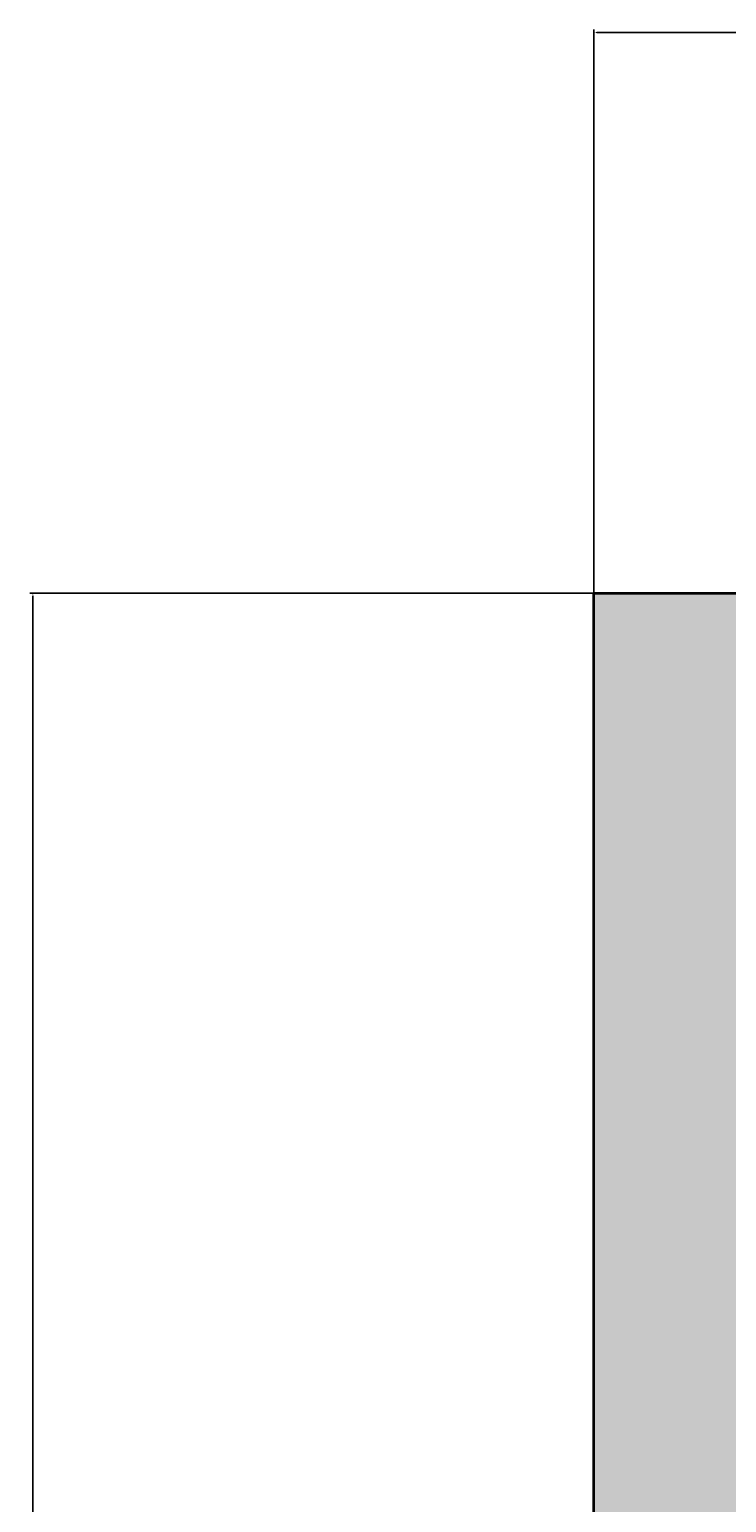
# Model space of a CAD drawing. Units: inches. Extents: x 2070 to 4408, y 1595 to 4269.
# Tile 12 of 20: x 2070 to 2111, y 2238 to 2325. Entities that reach past the tile are written whole.
import ezdxf

# ---------------------------------------------------------------- set-up
doc = ezdxf.new("R2010")
doc.units = ezdxf.units.IN
doc.layers.add('A-ANNO-DIMS', color=2, linetype='Continuous', lineweight=18)
doc.layers.add('A-WALL', color=7, linetype='Continuous', lineweight=35)
doc.layers.add('A-WALL-PATT', color=18, linetype='Continuous', lineweight=13, true_color=0x000000)
doc.styles.get("Standard").update_dxf_attribs({"font": 'arial.ttf'})
doc.dimstyles.get("Standard").update_dxf_attribs({"dimtxt": 0.18, "dimasz": 0.18, "dimexe": 0.18, "dimexo": 0.0625, "dimgap": 0.09, "dimtad": 0, "dimtih": 1, "dimtoh": 1, "dimdec": 4, "dimzin": 0, "dimdsep": 46, "dimtxsty": 'Standard', "dimcen": 0.09, "dimadec": 0, "dimazin": 0, "dimtfac": 1, "dimtdec": 4, "dimtofl": 0, "dimtmove": 0, "dimatfit": 3, "dimfxl": 1, "dimtolj": 1, "dimtzin": 0, "dimarcsym": 0})

# ---------------------------------------------------------------- blocks, each defined once
blk = doc.blocks.new('*D23')
at = {"layer": 'A-ANNO-DIMS', "color": 0, "lineweight": -2, "transparency": 16777216}
for p, q in [((2103.196, 2291.462), (2103.196, 2324.76)), ((2455.196, 2291.462), (2455.196, 2324.76)), ((2103.376, 2324.579), (2278.908, 2324.579)), ((2455.016, 2324.579), (2279.484, 2324.579))]:
    blk.add_line(p, q, dxfattribs=at)
at = {"layer": 'A-ANNO-DIMS', "color": 0, "transparency": 16777216}
for points in [[(2103.376, 2324.61), (2103.376, 2324.55), (2103.196, 2324.579)], [(2455.016, 2324.61), (2455.016, 2324.55), (2455.196, 2324.579)]]:
    blk.add_solid(points, dxfattribs=at)
at = {"layer": 'Defpoints', "color": 0, "transparency": 16777216}
for p in [(2455.196, 2324.579), (2103.196, 2291.399), (2455.196, 2291.399)]:
    blk.add_point(p, dxfattribs=at)
at = {"layer": 'A-ANNO-DIMS', "color": 0, "transparency": 16777216, "insert": (2279.196, 2324.579), "char_height": 0.18, "attachment_point": 5}
blk.add_mtext('\\A1;352', dxfattribs=at)
blk = doc.blocks.new('*D24')
at = {"layer": 'A-ANNO-DIMS', "color": 0, "lineweight": -2, "transparency": 16777216}
for p, q in [((2103.133, 2291.4), (2069.836, 2291.4)), ((2070.016, 2291.22), (2070.016, 1960.081)), ((2070.016, 1628.58), (2070.016, 1959.718)), ((2336.133, 1628.4), (2069.836, 1628.4))]:
    blk.add_line(p, q, dxfattribs=at)
at = {"layer": 'A-ANNO-DIMS', "color": 0, "transparency": 16777216}
for points in [[(2069.986, 2291.22), (2070.046, 2291.22), (2070.016, 2291.4)], [(2069.986, 1628.58), (2070.046, 1628.58), (2070.016, 1628.4)]]:
    blk.add_solid(points, dxfattribs=at)
at = {"layer": 'Defpoints', "color": 0, "transparency": 16777216}
for p in [(2070.016, 2291.4), (2103.196, 2291.4), (2336.196, 1628.4)]:
    blk.add_point(p, dxfattribs=at)
at = {"layer": 'A-ANNO-DIMS', "color": 0, "transparency": 16777216, "insert": (2070.016, 1959.899), "char_height": 0.18, "attachment_point": 5}
blk.add_mtext('\\A1;663', dxfattribs=at)

msp = doc.modelspace()

# ---------------------------------------------------------------- hatches: boundary and pattern name
at = {"layer": 'A-WALL-PATT'}
h = msp.add_hatch(color=256, dxfattribs=at)
h.dxf.hatch_style = 1
h.paths.add_polyline_path([(2346.196, 2218.3995), (2346.196, 2282.3995), (2340.196, 2282.3995), (2340.196, 2212.3995), (2345.5866, 2212.3995), (2346.196, 2212.3995)], flags=0)
h.paths.add_polyline_path([(2245.196, 2282.3995), (2239.196, 2282.3995), (2239.196, 2186.3995), (2244.5866, 2186.3995), (2245.196, 2186.3995)], flags=0)
h.paths.add_polyline_path([(2340.196, 2230.6455), (2245.196, 2230.6455), (2245.196, 2224.6455), (2340.196, 2224.6455)], flags=0)
h.paths.add_polyline_path([(2245.196, 2150.3995), (2239.196, 2150.3995), (2164.4362, 2150.3995), (2164.4362, 2144.3995), (2239.196, 2144.3995), (2239.196, 2086.3995), (2239.196, 2067.2711), (2244.5866, 2067.2711), (2245.196, 2067.2711), (2245.196, 2144.3995)], flags=0)
h.paths.add_polyline_path([(2346.196, 2176.3995), (2340.196, 2176.3995), (2340.196, 2086.3995), (2346.196, 2086.3995), (2346.196, 2125.318)], flags=0)
h.paths.add_polyline_path([(2446.196, 2086.3995), (2346.196, 2086.3995), (2340.196, 2086.3995), (2340.196, 2080.3995), (2446.196, 2080.3995)], flags=0)
h.paths.add_polyline_path([(2455.196, 2291.3995), (2103.196, 2291.3995), (2103.196, 1699.3995), (2336.196, 1699.3995), (2336.196, 1628.3995), (2345.196, 1628.3995), (2446.196, 1628.3995), (2454.8846, 1628.3995), (2454.8846, 1699.3995)])
h.paths.add_polyline_path([(2446.196, 2282.3995), (2446.196, 2218.3995), (2446.196, 2212.3995), (2446.196, 2086.3995), (2446.196, 2080.3995), (2446.196, 1708.3995), (2446.196, 1637.3995), (2345.196, 1637.3995), (2345.196, 1699.3995), (2345.196, 1708.3995), (2336.196, 1708.3995), (2112.196, 1708.3995), (2112.196, 2282.3995), (2239.196, 2282.3995), (2245.196, 2282.3995), (2356.196, 2282.3995)], flags=16)
h.paths.add_polyline_path([(2245.196, 2150.3995), (2245.196, 2144.3995), (2245.196, 2067.2711), (2244.5866, 2067.2711), (2239.196, 2067.2711), (2239.196, 2065.6988), (2203.2929, 2065.6988, 0.4014527), (2239.196, 2031.3337), (2244.5866, 2031.3337), (2245.196, 2031.2711), (2245.196, 1924.1525), (2239.196, 1924.1525), (2239.196, 1922.5803), (2203.2929, 1922.5803, 0.4014527), (2239.196, 1888.2151), (2244.5866, 1888.2151), (2245.196, 1888.1525), (2245.196, 1748.3995), (2339.196, 1748.4621, -0.4014527), (2303.2929, 1782.8272), (2303.2585, 1782.8272), (2303.2585, 1784.3995), (2339.196, 1784.3995), (2339.196, 1877.2067), (2291.196, 1877.2067), (2291.196, 1883.2067), (2291.196, 1946.3995), (2291.196, 1952.3995), (2291.196, 2086.3995), (2297.196, 2086.3995), (2302.196, 2086.3995), (2302.196, 2081.0259), (2303.7633, 2081.0259), (2303.7633, 2080.3995), (2338.0148, 2080.3995, 0.0043713), (2338.0203, 2081.0259), (2338.0203, 2086.3995), (2340.196, 2086.3995), (2340.196, 2176.4621), (2345.5866, 2176.4621, 0.4014527), (2381.4896, 2210.8272), (2345.5866, 2210.8272), (2345.5866, 2212.3995), (2340.196, 2212.3995), (2340.196, 2224.6455), (2245.196, 2224.6455), (2245.196, 2186.3995), (2244.5866, 2186.3995), (2239.196, 2186.3995), (2239.196, 2184.8272), (2203.2929, 2184.8272, 0.4014527), (2239.196, 2150.4621), (2244.5866, 2150.4621)], flags=0)
h.paths.add_polyline_path([(2346.196, 2282.3995), (2346.196, 2218.3995), (2377.1813, 2218.3995), (2377.1813, 2212.3995), (2346.196, 2212.3995), (2345.5866, 2212.3995), (2340.196, 2212.3995), (2340.196, 2224.6455), (2245.196, 2224.6455), (2245.196, 2230.6455), (2245.196, 2282.3995), (2292.696, 2256.5225), (2340.196, 2282.3995)], flags=0)
h.paths.add_polyline_path([(2346.196, 2086.3995), (2340.196, 2086.3995), (2340.196, 2080.3995), (2446.196, 2080.3995), (2431.196, 2016.3995), (2446.196, 1952.3995), (2412.196, 1952.3995), (2412.196, 2080.3995), (2340.196, 2080.3995), (2340.196, 2086.3995), (2340.196, 2176.3995), (2346.196, 2176.3995), (2346.196, 2125.318)], flags=0)
h.paths.add_polyline_path([(2186.508, 2270.0471, -0.0375529), (2186.9712, 2269.8581), (2186.9164, 2270.112, -0.0275912)], flags=0)
h.paths.add_polyline_path([(2183.955, 2273.7766, 1), (2188.2945, 2273.7766, 1)], flags=0)
h.paths.add_polyline_path([(2142.5261, 2274.6158, -0.0370754), (2142.5672, 2275.1696), (2142.5672, 2276.826), (2119.8759, 2276.826), (2119.8759, 2263.0962), (2140.4332, 2263.0962), (2142.5672, 2263.0962), (2142.5672, 2274.0621, -0.0370754)], flags=0)
h.paths.add_polyline_path([(2209.8974, 2263.0962), (2209.8974, 2262.2079), (2190.8042, 2262.2079), (2190.8042, 2263.0962)], flags=0)
h.paths.add_polyline_path([(2210.6382, 2276.1833), (2210.6382, 2263.9844), (2190.2185, 2263.9844), (2190.2185, 2276.1833)], flags=0)
h.paths.add_polyline_path([(2188.4362, 2273.7766, -1), (2183.8133, 2273.7766, -1)], flags=0)
h.paths.add_polyline_path([(2245.196, 2150.3995), (2245.196, 2144.3995), (2245.196, 2067.2711), (2239.196, 2067.2711), (2239.196, 2080.3995), (2172.196, 2080.3995), (2172.196, 2000.3995), (2239.196, 2000.3995), (2239.196, 1940.3995), (2159.0187, 1940.3995), (2123.0187, 1940.3995), (2112.196, 1940.3995), (2112.196, 1946.3995), (2123.0187, 1946.3995), (2123.0187, 1982.2238), (2124.586, 1982.2238), (2124.586, 1982.1895, -0.4014527), (2158.8429, 1946.3995), (2159.0187, 1946.3995), (2239.196, 1946.3995), (2239.196, 1994.3995), (2112.196, 1994.3995), (2112.196, 2000.3995), (2139.196, 2040.3995), (2112.196, 2080.3995), (2112.196, 2086.3995), (2239.196, 2086.3995), (2239.196, 2144.3995), (2209.5809, 2144.3995), (2209.5809, 2136.3995), (2203.0809, 2136.3995), (2205.0809, 2130.3996, -0.7025712), (2199.081, 2116.3995, -0.7025621), (2193.0809, 2130.3994), (2195.0809, 2136.3995), (2192.0809, 2136.3995), (2192.0809, 2134.8995), (2189.0809, 2134.8995), (2189.0809, 2135.8995), (2191.0809, 2135.8995), (2191.0809, 2136.3995), (2188.5809, 2136.3995), (2188.5809, 2144.3995), (2164.2481, 2144.3995, -0.3938585), (2130.0035, 2109.5491), (2130.0035, 2109.5147), (2128.4362, 2109.5147), (2128.4362, 2144.3995), (2112.196, 2144.3995), (2112.196, 2150.3995), (2128.4362, 2150.3995), (2128.4362, 2150.7127), (2164.4362, 2150.7127), (2164.4362, 2150.3995), (2239.196, 2150.3995)], flags=0)
h.paths.add_polyline_path([(2188.2075, 2266.8735), (2188.2075, 2211.8632, -0.4142136), (2185.4833, 2209.1391), (2146.7995, 2209.1391, -0.4142136), (2144.0754, 2211.8632), (2144.0754, 2266.8735, -0.4142136), (2146.7995, 2269.5976), (2185.4833, 2269.5976, -0.4142136)], flags=0)
h.paths.add_polyline_path([(2185.0844, 2273.7766, -1), (2187.1651, 2273.7766, -1)], flags=0)
h.paths.add_polyline_path([(2182.0486, 2259.2932), (2168.0953, 2259.2932), (2168.0953, 2260.8424), (2163.7261, 2260.8424), (2163.7261, 2259.2932), (2149.7727, 2259.2932), (2149.7727, 2266.3352), (2163.7261, 2266.3352), (2163.7261, 2261.9839), (2168.0953, 2261.9839), (2168.0953, 2266.3352), (2182.0486, 2266.3352)], flags=0)
h.paths.add_polyline_path([(2148.2585, 2250.2051), (2153.0615, 2241.8861, 0.3980705)], flags=0)
h.paths.add_polyline_path([(2162.7572, 2247.2885), (2153.1461, 2241.7396), (2148.1083, 2250.4653), (2157.7194, 2256.0142)], flags=0)
h.paths.add_polyline_path([(2162.6726, 2247.4351, -0.392862), (2157.8415, 2255.6313), (2157.6431, 2255.6313), (2157.8696, 2255.7541)], flags=0)
h.paths.add_polyline_path([(2164.2604, 2145.339), (2164.4362, 2144.3995), (2164.4362, 2150.3995), (2164.2604, 2150.7127)], flags=0)
h.paths.add_polyline_path([(2208.5809, 2142.6495), (2208.5809, 2138.3995, -0.4142136), (2207.8309, 2137.3995), (2190.5809, 2137.3995, -0.4142136), (2189.5809, 2138.1495), (2189.5809, 2142.3995, -0.4142136), (2190.3309, 2143.3995), (2207.5809, 2143.3995, -0.4142136)], flags=0)
h.paths.add_polyline_path([(2147.957, 2229.9119), (2154.7494, 2223.1195, 0.3980705)], flags=0)
h.paths.add_polyline_path([(2162.7165, 2230.8473), (2154.8691, 2222.9998), (2147.7446, 2230.1244), (2155.592, 2237.9718)], flags=0)
h.paths.add_polyline_path([(2162.5969, 2230.9669, -0.3980705), (2155.8044, 2237.7594)], flags=0)
h.paths.add_polyline_path([(2391.8776, 2049.9192), (2408.5766, 2049.9192), (2408.5766, 2033.2202), (2408.5766, 1983.123), (2408.5766, 1966.4239), (2391.8776, 1966.4239), (2391.8776, 1983.123), (2341.7804, 1983.123), (2341.7804, 2033.2202), (2391.8776, 2033.2202)], flags=0)
h.paths.add_polyline_path([(2144.1055, 2274.6158, 1), (2148.445, 2274.6158, 1)], flags=0)
h.paths.add_polyline_path([(2148.5867, 2274.6158, -1), (2143.9638, 2274.6158, -1)], flags=0)
h.paths.add_polyline_path([(2145.2349, 2274.6158, -1), (2147.3156, 2274.6158, -1)], flags=0)
edge = h.paths.add_edge_path(flags=0)
edge.add_ellipse((2400.5951, 2040.9436), major_axis=(-4.5109, 0), ratio=0.9754478, start_angle=180, end_angle=270, ccw=False)
edge.add_ellipse((2400.5951, 2040.9436), major_axis=(-4.5109, 0), ratio=0.9754478, start_angle=90, end_angle=180, ccw=False)
edge.add_ellipse((2400.5951, 2040.9436), major_axis=(-4.5109, 0), ratio=0.9754478, start_angle=0, end_angle=90, ccw=False)
edge.add_ellipse((2400.5951, 2040.9436), major_axis=(-4.5109, 0), ratio=0.9754478, start_angle=270, end_angle=360, ccw=False)
h.paths.add_polyline_path([(2199.0809, 2117.3995, -0.7345297), (2195.0809, 2130.3995), (2203.081, 2130.3995, -0.7345333)], flags=0)
h.paths.add_polyline_path([(2141.9147, 2276.0353), (2141.9147, 2263.9844), (2120.4685, 2263.9844), (2120.4685, 2276.0353)], flags=0)
h.paths.add_polyline_path([(2138.4481, 2273.4072), (2138.4481, 2266.7226), (2133.2801, 2266.7226), (2133.2801, 2273.4072)], flags=0)
h.paths.add_polyline_path([(2137.9691, 2272.9175), (2137.9691, 2272.204), (2135.4229, 2272.204), (2135.4229, 2271.6329), (2135.3221, 2270.1051), (2135.3221, 2269.0265), (2135.4229, 2268.6811), (2135.4229, 2267.2011), (2133.7212, 2267.2011), (2133.7212, 2268.6811), (2133.7983, 2269.9587), (2133.7983, 2271.2758), (2133.7212, 2271.6329), (2133.7212, 2273.0065), (2135.717, 2273.0065), (2135.717, 2272.9175)], flags=0)
h.paths.add_polyline_path([(2137.9215, 2271.8264), (2137.9215, 2271.3786), (2137.5182, 2271.3786), (2136.9355, 2271.3786), (2136.3529, 2271.3786), (2135.7703, 2271.3786), (2135.7703, 2271.8264), (2136.1736, 2271.8264), (2136.7562, 2271.8264), (2137.3389, 2271.8264)], flags=0)
h.paths.add_polyline_path([(2137.9215, 2271.692), (2137.5182, 2271.692), (2136.9355, 2271.513), (2137.3389, 2271.513)], flags=0)
h.paths.add_polyline_path([(2136.3529, 2271.692), (2135.7703, 2271.513), (2136.1736, 2271.513), (2136.7562, 2271.692)], flags=0)
h.paths.add_polyline_path([(2137.9215, 2271.513), (2137.5182, 2271.513), (2136.7562, 2271.747), (2136.7562, 2271.692), (2137.3389, 2271.692)], flags=0)
h.paths.add_polyline_path([(2137.8207, 2270.4664), (2137.8207, 2270.0971), (2137.8207, 2269.627), (2137.8207, 2269.1569), (2137.8207, 2268.6868), (2137.3837, 2268.6868), (2136.6442, 2268.6868), (2135.9271, 2268.6868), (2135.9271, 2269.0562), (2135.9271, 2269.5263), (2135.9271, 2269.9963), (2135.9271, 2270.4664), (2136.3641, 2270.4664), (2137.0812, 2270.4664)], flags=0)
h.paths.add_polyline_path([(2137.3837, 2269.627), (2137.8207, 2269.627), (2137.8207, 2269.5263), (2137.3837, 2269.5263), (2137.3837, 2269.1569), (2137.8207, 2269.1569), (2137.3837, 2269.0562), (2137.3837, 2268.6868), (2137.0812, 2268.6868), (2137.0812, 2269.0562), (2136.6442, 2269.0562), (2136.6442, 2268.6868), (2136.3641, 2268.6868), (2136.3641, 2269.0562), (2135.9271, 2269.0562), (2135.9271, 2269.1569), (2136.3641, 2269.1569), (2136.3641, 2269.5263), (2135.9271, 2269.5263), (2135.9271, 2269.627), (2136.3641, 2269.627), (2136.3641, 2269.9963), (2135.9271, 2269.9963), (2136.3641, 2270.0971), (2136.3641, 2270.4664), (2136.6442, 2270.4664), (2136.6442, 2270.0971), (2137.0812, 2270.0971), (2137.0812, 2270.4664), (2137.3837, 2270.4664), (2137.3837, 2270.0971), (2137.8207, 2270.0971), (2137.3837, 2269.9963)], flags=0)
h.paths.add_polyline_path([(2137.5182, 2271.8264), (2137.5182, 2271.692), (2137.3389, 2271.3786), (2137.3389, 2271.513)], flags=0)
h.paths.add_polyline_path([(2137.8179, 2267.8138), (2137.8179, 2267.6879), (2137.1876, 2267.6879), (2136.4733, 2267.6879), (2135.759, 2267.6879), (2135.759, 2267.8138), (2136.3893, 2267.8138), (2137.1036, 2267.8138)], flags=0)
h.paths.add_polyline_path([(2137.0812, 2269.9963), (2137.0812, 2269.627), (2137.0812, 2269.1569), (2136.6442, 2269.1569), (2136.6442, 2269.5263), (2136.6442, 2269.9963)], flags=0)
h.paths.add_polyline_path([(2136.3529, 2271.8264), (2136.3529, 2271.692), (2136.1736, 2271.3786), (2136.1736, 2271.513)], flags=0)
h.paths.add_polyline_path([(2136.4733, 2267.8138), (2136.4733, 2267.6879), (2136.3893, 2267.6879), (2136.3893, 2267.8138)], flags=0)
h.paths.add_polyline_path([(2407.9087, 2032.5522), (2407.9087, 1983.7909), (2359.81, 1983.7909, -0.0091279), (2359.0575, 1983.7909), (2342.4483, 1983.7909), (2342.4483, 2032.5522)], flags=0)
h.paths.add_polyline_path([(2389.1838, 2023.1358), (2353.7856, 2023.1358), (2353.7856, 1985.4867, -0.0921038), (2350.2788, 1988.655), (2350.2788, 2026.6426), (2389.1838, 2026.6426)], flags=0)
h.paths.add_polyline_path([(2352.6166, 2024.3048), (2351.4477, 2024.3048), (2351.4477, 2025.4737), (2352.6166, 2025.4737)], flags=0)
h.paths.add_polyline_path([(2399.6319, 2026.7589), (2404.3661, 2026.7589, -0.4142136), (2407.0379, 2024.087), (2407.0379, 2013.4908, -0.4142136), (2404.3661, 2010.819), (2399.6319, 2010.819, -0.4142136), (2396.96, 2013.4908), (2396.96, 2024.087, -0.4142136)], flags=0)
h.paths.add_polyline_path([(2399.6319, 2026.0909), (2404.3661, 2026.0909, -0.4142136), (2406.37, 2024.087), (2406.37, 2013.4908, -0.4142136), (2404.3661, 2011.487), (2399.6319, 2011.487, -0.4142136), (2397.628, 2013.4908), (2397.628, 2024.087, -0.4142136)], flags=0)
h.paths.add_polyline_path([(2399.6319, 2002.3217), (2404.3661, 2002.3217, -0.4142136), (2407.0379, 1999.6498), (2407.0379, 1989.0536, -0.4142136), (2404.3661, 1986.3818), (2399.6319, 1986.3818, -0.4142136), (2396.96, 1989.0536), (2396.96, 1999.6498, -0.4142136)], flags=0)
h.paths.add_polyline_path([(2399.6319, 2001.6537), (2404.3661, 2001.6537, -0.4142136), (2406.37, 1999.6498), (2406.37, 1989.0536, -0.4142136), (2404.3661, 1987.0497), (2399.6319, 1987.0497, -0.4142136), (2397.628, 1989.0536), (2397.628, 1999.6498, -0.4142136)], flags=0)
edge = h.paths.add_edge_path(flags=0)
edge.add_ellipse((2400.5951, 1975.3996), major_axis=(-4.5109, 0), ratio=0.9754478, start_angle=-180, end_angle=-90, ccw=False)
edge.add_ellipse((2400.5951, 1975.3996), major_axis=(-4.5109, 0), ratio=0.9754478, start_angle=90, end_angle=180, ccw=False)
edge.add_ellipse((2400.5951, 1975.3996), major_axis=(-4.5109, 0), ratio=0.9754478, start_angle=0, end_angle=90, ccw=False)
edge.add_ellipse((2400.5951, 1975.3996), major_axis=(-4.5109, 0), ratio=0.9754478, start_angle=-90, end_angle=0, ccw=False)
h.paths.add_polyline_path([(2345.196, 1910.3995), (2366.4386, 1910.3995), (2366.4386, 1925.4555), (2392.3856, 1925.4555), (2392.3856, 1933.5025), (2400.1399, 1925.4555), (2392.3856, 1919.8795), (2392.3856, 1925.4555), (2366.4386, 1925.4555), (2366.4386, 1910.3995), (2381.196, 1910.3995), (2405.196, 1910.3995), (2405.196, 1898.3995), (2446.196, 1898.3995), (2446.196, 1886.3995), (2405.196, 1886.3995), (2405.196, 1874.3995), (2446.196, 1874.3995), (2446.196, 1862.3995), (2405.196, 1862.3995), (2405.196, 1850.3995), (2446.196, 1850.3995), (2446.196, 1838.3995), (2405.196, 1838.3995), (2405.196, 1826.3995), (2446.196, 1826.3995), (2446.196, 1814.3995), (2405.196, 1814.3995), (2405.196, 1802.3995), (2446.196, 1802.3995), (2446.196, 1798.3995), (2446.196, 1792.3995), (2405.196, 1792.3995), (2405.196, 1910.3995), (2381.196, 1910.3995), (2381.196, 1792.3995), (2345.196, 1792.3995)], flags=0)
h.paths.add_polyline_path([(2333.0944, 1863.3993, -0.4142136), (2334.7225, 1861.7712), (2334.7225, 1859.329), (2335.2653, 1859.329, -0.4142136), (2337.4361, 1857.1582), (2337.4361, 1843.862, -0.4142136), (2335.2653, 1841.6911, -0.4142136), (2337.4361, 1839.5203), (2337.4361, 1827.5808, -0.4142136), (2335.2653, 1825.41, -0.4142136), (2337.4361, 1823.2392), (2337.4361, 1808.5862, -0.4142136), (2335.2653, 1806.4153), (2334.7225, 1806.4153), (2334.7225, 1803.9732, -0.4142136), (2333.0944, 1802.3451), (2317.356, 1802.3451), (2317.0846, 1802.3451, -0.4142136), (2315.7279, 1803.7018), (2315.7279, 1803.8646), (2313.8284, 1803.8646, -0.4142136), (2311.6576, 1806.0354), (2311.6576, 1823.2015, -0.395976), (2313.6834, 1825.3765, -0.433848), (2311.6576, 1827.2718), (2311.6576, 1839.761, -0.4142136), (2313.5571, 1841.6604), (2313.8284, 1841.6604), (2333.8159, 1841.6604, -0.0421362), (2334.1798, 1841.6911, -0.4142136), (2332.009, 1843.862), (2332.009, 1857.1582, -0.4142136), (2334.1798, 1859.329), (2317.356, 1859.329), (2317.0846, 1859.329, -0.4142136), (2315.7279, 1860.6858), (2315.7279, 1862.0426, -0.4142136), (2317.0846, 1863.3993), (2317.356, 1863.3993)], flags=0)
h.paths.add_polyline_path([(2208.8475, 1848.9818), (2208.8475, 1840.9741, -0.4142136), (2207.0458, 1839.1724), (2206.5453, 1839.1721), (2206.5453, 1838.7218, -0.4098586), (2204.7704, 1836.9203), (2183.7501, 1836.9203, -0.418582), (2181.9216, 1838.7218), (2181.9216, 1839.1721), (2181.421, 1839.1724, -0.4142136), (2179.6193, 1840.9741), (2179.6193, 1848.6817, -0.4406442), (2185.1126, 1854.9874), (2203.3852, 1854.9874, -0.4570796)], flags=0)
h.paths.add_polyline_path([(2204.243, 1848.4815), (2204.243, 1848.4815, 0.4172533), (2202.2204, 1850.4833), (2186.2049, 1850.4833, 0.4111805), (2184.2237, 1848.4815), (2184.2237, 1848.4815, -0.4111807), (2186.2049, 1850.4833), (2202.2204, 1850.4833, -0.4172531)], flags=0)
h.paths.add_polyline_path([(2234.7177, 1830.228), (2234.7176, 1781.6047, -0.4142136), (2233.4381, 1780.3252), (2218.6064, 1780.3252, -0.4142136), (2217.8387, 1781.0929), (2217.8387, 1783.3961, -0.4142136), (2218.6064, 1784.1639), (2218.6065, 1796.9595, -0.4142136), (2219.886, 1798.239, -0.4142136), (2218.6065, 1799.5186), (2218.6065, 1812.3142, -0.4142136), (2219.8861, 1813.5938, -0.4142136), (2218.6065, 1814.8733), (2218.6065, 1827.6689, -0.4142136), (2217.8388, 1828.4367), (2217.8388, 1830.7399, -0.4142136), (2218.6065, 1831.5076), (2233.4382, 1831.5076, -0.4142136)], flags=0)
h.paths.add_polyline_path([(2230.6344, 1827.6689, -0.4142136), (2231.4021, 1826.9012), (2231.4021, 1784.9316, -0.4142136), (2230.6343, 1784.1639), (2221.1853, 1784.1639), (2221.1853, 1827.6689)], flags=0)
h.paths.add_polyline_path([(2222.7208, 1798.239), (2221.6971, 1798.239), (2221.6971, 1813.5938), (2222.7208, 1813.5938)], flags=0)
h.paths.add_polyline_path([(2206.5453, 1773.935), (2206.5453, 1773.4848), (2206.9457, 1773.4848), (2207.0458, 1773.4845, -0.4142136), (2208.8475, 1771.6827), (2208.8475, 1763.675, -0.4422243), (2203.6505, 1757.6695), (2185.3851, 1757.6695, -0.455084), (2179.6193, 1763.9752), (2179.6193, 1771.6827, -0.4142136), (2181.421, 1773.4845), (2181.421, 1773.4848), (2181.9216, 1773.4848), (2181.9216, 1773.935, -0.4098586), (2183.6965, 1775.7366), (2204.7167, 1775.7366, -0.418582)], flags=0)
h.paths.add_polyline_path([(2202.2619, 1762.1736), (2186.2464, 1762.1736, -0.4172531), (2184.2237, 1764.1754), (2184.2237, 1764.1754, 0.4172533), (2186.2464, 1762.1736), (2202.2619, 1762.1736, 0.4111805), (2204.243, 1764.1754), (2204.243, 1764.1754, -0.4111807)], flags=0)
h.paths.add_polyline_path([(2313.0034, 1713.1906), (2312.997, 1713.1697), (2313.0123, 1713.1612)], flags=0)
h.paths.add_polyline_path([(2305.7314, 1721.0488), (2305.6257, 1721.1994), (2305.4853, 1721.084)], flags=0)
h.paths.add_polyline_path([(2307.5562, 1726.1427), (2307.6186, 1726.1026), (2307.5737, 1726.0477), (2308.5692, 1720.6434), (2310.5345, 1721.2985), (2310.5721, 1721.411), (2310.6958, 1721.3523), (2313.8453, 1722.4021), (2314.9351, 1723.8033), (2314.9294, 1723.9165), (2315.0028, 1723.8903), (2313.874, 1722.4389), (2313.8697, 1722.4102), (2308.5692, 1720.6434), (2308.9864, 1720.122), (2309.0665, 1720.0971), (2309.053, 1720.0387), (2310.9235, 1717.7005), (2311.4182, 1717.6259), (2311.2918, 1717.2402), (2312.0655, 1716.2731), (2312.1081, 1716.2606), (2312.0969, 1716.2339), (2308.5692, 1720.6434), (2305.2249, 1717.745), (2305.232, 1717.704), (2305.1665, 1717.6944), (2308.5692, 1720.6434)], flags=0)
h.paths.add_polyline_path([(2288.2072, 1714.3431), (2288.2008, 1714.3222), (2288.216, 1714.3137)], flags=0)
h.paths.add_polyline_path([(2280.9352, 1722.2013), (2280.8295, 1722.3519), (2280.689, 1722.2365)], flags=0)
h.paths.add_polyline_path([(2282.76, 1727.2952), (2282.8224, 1727.2551), (2282.7775, 1727.2002), (2283.773, 1721.7959), (2285.7383, 1722.451), (2285.7759, 1722.5635), (2285.8995, 1722.5048), (2289.0491, 1723.5546), (2290.1389, 1724.9558), (2290.1332, 1725.069), (2290.2065, 1725.0428), (2289.0777, 1723.5915), (2289.0735, 1723.5628), (2283.773, 1721.7959), (2284.1901, 1721.2745), (2284.2703, 1721.2496), (2284.2567, 1721.1913), (2286.1273, 1718.8531), (2286.622, 1718.7785), (2286.4956, 1718.3927), (2287.2692, 1717.4256), (2287.3119, 1717.4131), (2287.3006, 1717.3864), (2283.773, 1721.7959), (2280.4286, 1718.8975), (2280.4357, 1718.8565), (2280.3703, 1718.8469), (2283.773, 1721.7959)], flags=0)
h.paths.add_polyline_path([(2302.0672, 1721.8694), (2301.8205, 1721.8572), (2301.7578, 1722.1787), (2299.415, 1724.5215), (2299.103, 1724.4694), (2299.0662, 1724.8703)], flags=0)
h.paths.add_polyline_path([(2264.5643, 1715.4956), (2264.5579, 1715.4747), (2264.5731, 1715.4662)], flags=0)
h.paths.add_polyline_path([(2257.2923, 1723.3538), (2257.1865, 1723.5044), (2257.0461, 1723.389)], flags=0)
h.paths.add_polyline_path([(2259.117, 1728.4477), (2259.1795, 1728.4077), (2259.1345, 1728.3527), (2260.13, 1722.9484), (2262.0954, 1723.6036), (2262.133, 1723.716), (2262.2566, 1723.6573), (2265.4061, 1724.7071), (2266.4959, 1726.1083), (2266.4902, 1726.2215), (2266.5636, 1726.1953), (2265.4348, 1724.744), (2265.4305, 1724.7153), (2260.13, 1722.9484), (2260.5472, 1722.427), (2260.6273, 1722.4022), (2260.6138, 1722.3438), (2262.4843, 1720.0056), (2262.979, 1719.931), (2262.8526, 1719.5452), (2263.6263, 1718.5781), (2263.6689, 1718.5656), (2263.6577, 1718.5389), (2260.13, 1722.9484), (2256.7857, 1720.05), (2256.7928, 1720.009), (2256.7273, 1719.9994), (2260.13, 1722.9484)], flags=0)
h.paths.add_polyline_path([(2277.2709, 1723.0219), (2277.0243, 1723.0097), (2276.9616, 1723.3312), (2274.6187, 1725.6741), (2274.3067, 1725.6219), (2274.27, 1726.0228)], flags=0)
h.paths.add_polyline_path([(2253.628, 1724.1744), (2253.3814, 1724.1622), (2253.3186, 1724.4838), (2250.9758, 1726.8266), (2250.6638, 1726.7744), (2250.627, 1727.1753)], flags=0)
h.paths.add_polyline_path([(2161.9194, 1715.4956), (2161.913, 1715.4747), (2161.9282, 1715.4662)], flags=0)
h.paths.add_polyline_path([(2154.6474, 1723.3538), (2154.5416, 1723.5044), (2154.4012, 1723.389)], flags=0)
h.paths.add_polyline_path([(2162.7899, 1724.744), (2162.7856, 1724.7153), (2157.4851, 1722.9484), (2157.9023, 1722.427), (2157.9824, 1722.4022), (2157.9689, 1722.3438), (2159.8394, 1720.0056), (2160.3341, 1719.931), (2160.2078, 1719.5452), (2160.9814, 1718.5781), (2161.024, 1718.5656), (2161.0128, 1718.5389), (2157.4851, 1722.9484), (2154.1408, 1720.05), (2154.1479, 1720.009), (2154.0824, 1719.9994), (2157.4851, 1722.9484), (2156.4721, 1728.4477), (2156.5346, 1728.4077), (2156.4896, 1728.3527), (2157.4851, 1722.9484), (2159.4505, 1723.6036), (2159.4881, 1723.716), (2159.6117, 1723.6573), (2162.7612, 1724.7071), (2163.851, 1726.1083), (2163.8453, 1726.2215), (2163.9187, 1726.1953)], flags=0)
h.paths.add_polyline_path([(2150.9831, 1724.1744), (2150.7365, 1724.1622), (2150.6738, 1724.4838), (2148.3309, 1726.8266), (2148.0189, 1726.7744), (2147.9822, 1727.1753)], flags=0)
h.paths.add_polyline_path([(2132.5099, 1716.6482), (2132.5035, 1716.6272), (2132.5187, 1716.6187)], flags=0)
h.paths.add_polyline_path([(2125.2379, 1724.5064), (2125.1322, 1724.6569), (2124.9917, 1724.5415)], flags=0)
h.paths.add_polyline_path([(2133.3804, 1725.8965), (2133.3762, 1725.8678), (2128.0757, 1724.101), (2128.4928, 1723.5795), (2128.5729, 1723.5547), (2128.5594, 1723.4963), (2130.43, 1721.1581), (2130.9246, 1721.0835), (2130.7983, 1720.6977), (2131.5719, 1719.7306), (2131.6146, 1719.7181), (2131.6033, 1719.6914), (2128.0757, 1724.101), (2124.7313, 1721.2025), (2124.7384, 1721.1615), (2124.6729, 1721.1519), (2128.0757, 1724.101), (2127.0626, 1729.6002), (2127.1251, 1729.5602), (2127.0801, 1729.5052), (2128.0757, 1724.101), (2130.041, 1724.7561), (2130.0786, 1724.8685), (2130.2022, 1724.8098), (2133.3517, 1725.8597), (2134.4415, 1727.2608), (2134.4358, 1727.3741), (2134.5092, 1727.3478)], flags=0)
h.paths.add_polyline_path([(2121.5736, 1725.3269), (2121.327, 1725.3148), (2121.2643, 1725.6363), (2118.9214, 1727.9791), (2118.6094, 1727.9269), (2118.5727, 1728.3279)], flags=0)
h.paths.add_polyline_path([(2433.3904, 1646.406), (2433.384, 1646.3851), (2433.3992, 1646.3766)], flags=0)
h.paths.add_polyline_path([(2426.1184, 1654.2642), (2426.0127, 1654.4148), (2425.8722, 1654.2994)], flags=0)
h.paths.add_polyline_path([(2427.9432, 1659.3581), (2428.0056, 1659.318), (2427.9606, 1659.2631), (2428.9562, 1653.8588), (2430.9215, 1654.514), (2430.9591, 1654.6264), (2431.0827, 1654.5677), (2434.2323, 1655.6175), (2435.322, 1657.0187), (2435.3163, 1657.1319), (2435.3897, 1657.1057), (2434.2609, 1655.6544), (2434.2567, 1655.6257), (2428.9562, 1653.8588), (2429.3733, 1653.3374), (2429.4534, 1653.3126), (2429.4399, 1653.2542), (2431.3105, 1650.916), (2431.8051, 1650.8414), (2431.6788, 1650.4556), (2432.4524, 1649.4885), (2432.4951, 1649.476), (2432.4838, 1649.4493), (2428.9562, 1653.8588), (2425.6118, 1650.9604), (2425.6189, 1650.9194), (2425.5535, 1650.9098), (2428.9562, 1653.8588)], flags=0)
h.paths.add_polyline_path([(2376.63, 1645.4912), (2376.6236, 1645.4703), (2376.6388, 1645.4617)], flags=0)
h.paths.add_polyline_path([(2369.358, 1653.3494), (2369.2523, 1653.5), (2369.1118, 1653.3845)], flags=0)
h.paths.add_polyline_path([(2371.1828, 1658.4432), (2371.2452, 1658.4032), (2371.2003, 1658.3482), (2372.1958, 1652.944), (2374.1611, 1653.5991), (2374.1987, 1653.7116), (2374.3224, 1653.6528), (2377.4719, 1654.7027), (2378.5617, 1656.1038), (2378.556, 1656.2171), (2378.6293, 1656.1908), (2377.5005, 1654.7395), (2377.4963, 1654.7108), (2372.1958, 1652.944), (2372.6129, 1652.4225), (2372.6931, 1652.3977), (2372.6795, 1652.3393), (2374.5501, 1650.0011), (2375.0448, 1649.9265), (2374.9184, 1649.5407), (2375.692, 1648.5737), (2375.7347, 1648.5611), (2375.7234, 1648.5344), (2372.1958, 1652.944), (2368.8514, 1650.0456), (2368.8586, 1650.0046), (2368.7931, 1649.995), (2372.1958, 1652.944)], flags=0)
h.paths.add_polyline_path([(2404.0947, 1645.0338), (2404.0883, 1645.0128), (2404.1035, 1645.0043)], flags=0)
h.paths.add_polyline_path([(2396.8227, 1652.892), (2396.717, 1653.0425), (2396.5765, 1652.9271)], flags=0)
h.paths.add_polyline_path([(2398.6475, 1657.9858), (2398.7099, 1657.9458), (2398.665, 1657.8908), (2399.6605, 1652.4866), (2401.6258, 1653.1417), (2401.6634, 1653.2541), (2401.7871, 1653.1954), (2404.9366, 1654.2453), (2406.0264, 1655.6464), (2406.0207, 1655.7596), (2406.094, 1655.7334), (2404.9652, 1654.2821), (2404.961, 1654.2534), (2399.6605, 1652.4866), (2400.0776, 1651.9651), (2400.1578, 1651.9403), (2400.1442, 1651.8819), (2402.0148, 1649.5437), (2402.5095, 1649.4691), (2402.3831, 1649.0833), (2403.1567, 1648.1162), (2403.1994, 1648.1037), (2403.1881, 1648.077), (2399.6605, 1652.4866), (2396.3162, 1649.5881), (2396.3233, 1649.5471), (2396.2578, 1649.5375), (2399.6605, 1652.4866)], flags=0)
h.paths.add_polyline_path([(2419.4532, 1658.0857), (2422.4541, 1655.0848), (2422.2075, 1655.0726), (2422.1448, 1655.3941), (2419.8019, 1657.737), (2419.4899, 1657.6848)], flags=0)
h.paths.add_polyline_path([(2390.1575, 1656.7135), (2393.1584, 1653.7125), (2392.9118, 1653.7004), (2392.8491, 1654.0219), (2390.5063, 1656.3647), (2390.1943, 1656.3125)], flags=0)
h.paths.add_polyline_path([(2362.6928, 1657.1709), (2365.6937, 1654.1699), (2365.4471, 1654.1578), (2365.3844, 1654.4793), (2363.0416, 1656.8221), (2362.7295, 1656.77)], flags=0)
h.paths.add_polyline_path([(2419.9523, 2037.8601), (2440.2872, 2037.8601), (2440.2872, 2047.1732), (2419.9523, 2047.1732)], flags=8)
h.paths.add_polyline_path([(2370.186, 1698.9005), (2413.6287, 1698.9005), (2413.6287, 1708.0908), (2370.186, 1708.0908)], flags=8)
h.paths.add_polyline_path([(2370.1656, 1708.5185), (2430.0857, 1708.5185), (2430.0857, 1717.8316), (2370.1656, 1717.8316)], flags=8)
h.paths.add_polyline_path([(2254.1469, 1788.1883), (2302.2471, 1788.1883), (2302.2471, 1797.3786), (2254.1469, 1797.3786)], flags=8)
h.paths.add_polyline_path([(2254.1264, 1797.8063), (2326.1448, 1797.8063), (2326.1448, 1807.1194), (2254.1264, 1807.1194)], flags=8)
h.paths.add_polyline_path([(2300.08, 1914.5069), (2338.861, 1914.5069), (2338.861, 1923.6972), (2300.08, 1923.6972)], flags=8)
h.paths.add_polyline_path([(2300.0595, 1924.1249), (2331.5882, 1924.1249), (2331.5882, 1933.438), (2300.0595, 1933.438)], flags=8)
h.paths.add_polyline_path([(2176.6905, 1716.4567), (2224.1441, 1716.4567), (2224.1441, 1725.647), (2176.6905, 1725.647)], flags=8)
h.paths.add_polyline_path([(2176.67, 1726.0747), (2245.9176, 1726.0747), (2245.9176, 1735.3878), (2176.67, 1735.3878)], flags=8)
h.paths.add_polyline_path([(2339.997, 2039.7696), (2388.1034, 2039.7696), (2388.1034, 2048.9661), (2339.997, 2048.9661)], flags=8)
h.paths.add_polyline_path([(2339.9776, 2049.3928), (2388.7204, 2049.3928), (2388.7204, 2058.7059), (2339.9776, 2058.7059)], flags=8)
h.paths.add_polyline_path([(2366.0063, 2161.3825), (2409.449, 2161.3825), (2409.449, 2170.5728), (2366.0063, 2170.5728)], flags=8)
h.paths.add_polyline_path([(2365.9868, 2171.0016), (2405.879, 2171.0016), (2405.879, 2180.3085), (2365.9868, 2180.3085)], flags=8)
h.paths.add_polyline_path([(2366.0102, 2247.0726), (2407.12, 2247.0726), (2407.12, 2256.263), (2366.0102, 2256.263)], flags=8)
h.paths.add_polyline_path([(2365.9897, 2256.6906), (2397.9686, 2256.6906), (2397.9686, 2266.0037), (2365.9897, 2266.0037)], flags=8)
h.paths.add_polyline_path([(2271.8465, 2102.7885), (2307.6541, 2102.7885), (2307.6541, 2111.9849), (2271.8465, 2111.9849)], flags=8)
h.paths.add_polyline_path([(2271.8281, 2112.4126), (2304.2673, 2112.4126), (2304.2673, 2121.7196), (2271.8281, 2121.7196)], flags=8)
h.paths.add_polyline_path([(2141.6408, 2187.5934), (2182.108, 2187.5934), (2182.108, 2196.7837), (2141.6408, 2196.7837)], flags=8)
h.paths.add_polyline_path([(2141.6203, 2197.2114), (2190.3631, 2197.2114), (2190.3631, 2206.5245), (2141.6203, 2206.5245)], flags=8)
h.paths.add_polyline_path([(2165.7271, 2103.039), (2211.5027, 2103.039), (2211.5027, 2112.2293), (2165.7271, 2112.2293)], flags=8)
h.paths.add_polyline_path([(2165.7077, 2112.658), (2185.1033, 2112.658), (2185.1033, 2121.965), (2165.7077, 2121.965)], flags=8)
h.paths.add_polyline_path([(2174.945, 2048.0789), (2211.3973, 2048.0789), (2211.3973, 2057.2693), (2174.945, 2057.2693)], flags=8)
h.paths.add_polyline_path([(2174.9256, 2057.698), (2194.3212, 2057.698), (2194.3212, 2067.0049), (2174.9256, 2067.0049)], flags=8)
h.paths.add_polyline_path([(2164.8305, 1965.8394), (2202.9649, 1965.8394), (2202.9649, 1975.0297), (2164.8305, 1975.0297)], flags=8)
h.paths.add_polyline_path([(2164.8111, 1975.4584), (2184.2067, 1975.4584), (2184.2067, 1984.7654), (2164.8111, 1984.7654)], flags=8)
h.paths.add_polyline_path([(2133.0392, 1862.086), (2173.5065, 1862.086), (2173.5065, 1871.2763), (2133.0392, 1871.2763)], flags=8)
h.paths.add_polyline_path([(2133.0709, 1871.8585), (2157.0382, 1871.8585), (2157.0382, 1880.8585), (2133.0709, 1880.8585)], flags=8)
h.paths.add_polyline_path([(2406.4423, 1923.5541), (2418.8209, 1923.5541), (2418.8209, 1932.7199), (2406.4423, 1932.7199)], flags=8)

# ---------------------------------------------------------------- linework, layer by layer
at = {"layer": 'A-WALL'}
msp.add_lwpolyline([(2336.196, 1699.3995), (2103.196, 1699.3995), (2103.196, 2291.3995), (2455.196, 2291.3995), (2455.196, 1699.3995), (2454.8846, 1699.3995)], dxfattribs=at)

# ---------------------------------------------------------------- dimensions: what is measured, and where the dimension line sits
at = {"layer": 'A-ANNO-DIMS'}
dim = msp.add_linear_dim(base=(2455.196, 2324.5795), p1=(2103.196, 2291.3995), p2=(2455.196, 2291.3995), dimstyle='Standard', override={"dimdec": 0, "dimlfac": 1, "dimrnd": 0, "dimzin": 0, "dimdsep": 46, "dimlunit": 2}, dxfattribs=at)
dim.commit()
dim.dimension.update_dxf_attribs({"geometry": '*D23', "text_midpoint": (2279.196, 2324.5795)})
dim = msp.add_linear_dim(base=(2070.016, 2291.3995), p1=(2336.196, 1628.3995), p2=(2103.196, 2291.3995), angle=90, dimstyle='Standard', override={"dimdec": 0, "dimlfac": 1, "dimrnd": 0, "dimzin": 0, "dimdsep": 46, "dimlunit": 2}, dxfattribs=at)
dim.commit()
dim.dimension.update_dxf_attribs({"geometry": '*D24', "text_midpoint": (2070.016, 1959.8995)})

doc.saveas('drawing.dxf')
